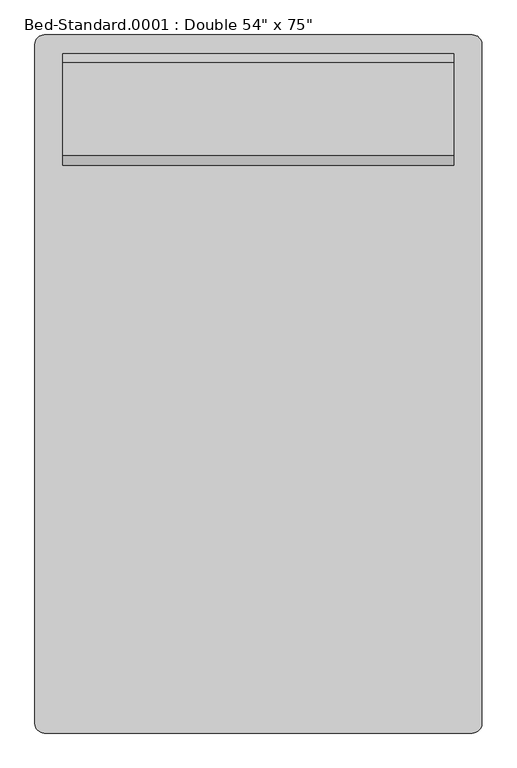
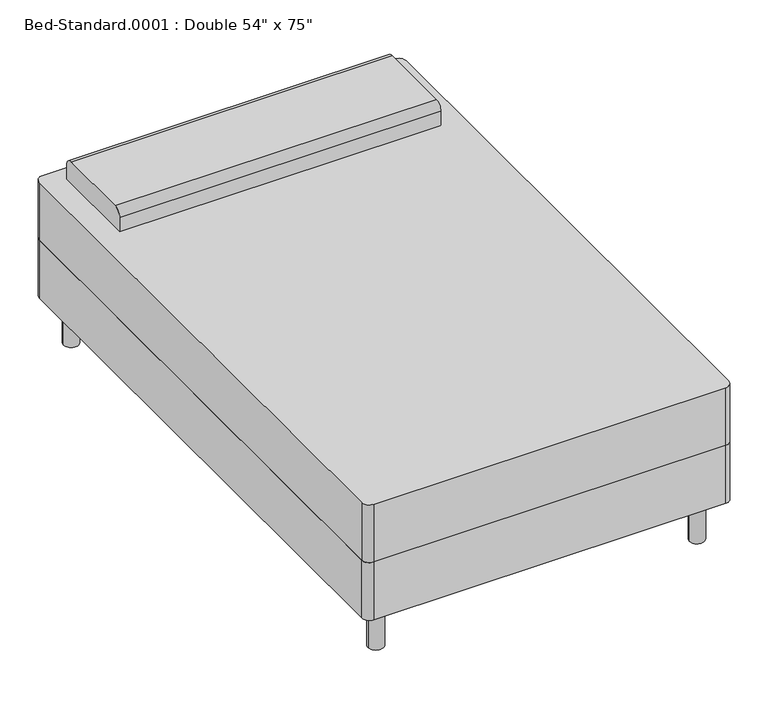
"""IFC4 building model written with IfcOpenShell, lengths in millimetres: furniture geometry."""

from ifc_helpers import new_model, si_unit, point, frame, frame_2d, origin, origin_with_axes, place, context, project, spatial, polyline, circle_curve, trimmed, segment, composite_curve, outline, extrude, source, transform, mapped, element, save


def furniture_4e05012c(model_context):
    return source(origin(), model_context, "Body", "SweptSolid", [
        extrude(outline(composite_curve([segment(polyline([(-338.1114754, -972.695082), (-338.1114754, 881.504918)]), True, "CONTINUOUS"), segment(trimmed(circle_curve(frame_2d((-312.7114754, 881.504918)), 25.4), [point((-338.1114754, 881.504918))], [point((-312.7114754, 906.904918))], False, "CARTESIAN"), True, "CONTINUOUS"), segment(polyline([(-312.7114754, 906.904918), (855.6885246, 906.904918)]), True, "CONTINUOUS"), segment(trimmed(circle_curve(frame_2d((855.6885246, 881.504918)), 25.4), [point((855.6885246, 906.904918))], [point((881.0885246, 881.504918))], False, "CARTESIAN"), True, "CONTINUOUS"), segment(polyline([(881.0885246, 881.504918), (881.0885246, -972.695082)]), True, "CONTINUOUS"), segment(trimmed(circle_curve(frame_2d((855.6885246, -972.695082)), 25.4), [point((881.0885246, -972.695082))], [point((855.6885246, -998.095082))], False, "CARTESIAN"), True, "CONTINUOUS"), segment(polyline([(855.6885246, -998.095082), (-312.7114754, -998.095082)]), True, "CONTINUOUS"), segment(trimmed(circle_curve(frame_2d((-312.7114754, -972.695082)), 25.4), [point((-312.7114754, -998.095082))], [point((-338.1114754, -972.695082))], False, "CARTESIAN"), True, "CONTINUOUS")], self_intersect=False)), frame((0.0, 0.0, 152.4), z_axis=(0.0, 0.0, 1.0), x_axis=(1.0, 0.0, 0.0)), (0.0, 0.0, 1.0), 203.2),
        extrude(outline(composite_curve([segment(polyline([(551.304918, 558.8), (551.304918, 609.6)]), True, "CONTINUOUS"), segment(trimmed(circle_curve(frame_2d((576.704918, 609.6)), 25.4), [point((551.304918, 609.6))], [point((576.704918, 635.0))], False, "CARTESIAN"), True, "CONTINUOUS"), segment(polyline([(576.704918, 635.0), (830.704918, 635.0)]), True, "CONTINUOUS"), segment(trimmed(circle_curve(frame_2d((830.704918, 609.6)), 25.4), [point((830.704918, 635.0))], [point((856.104918, 609.6))], False, "CARTESIAN"), True, "CONTINUOUS"), segment(polyline([(856.104918, 609.6), (856.104918, 558.8), (551.304918, 558.8)]), True, "CONTINUOUS")], self_intersect=False)), frame((-261.9114754, 0.0, 0.0), z_axis=(1.0, 0.0, 0.0), x_axis=(0.0, 1.0, 0.0)), (0.0, 0.0, 1.0), 1066.8),
        extrude(outline(composite_curve([segment(trimmed(circle_curve(frame_2d((-261.9114754, 830.704918)), 25.4), [point((-287.3114754, 830.704918))], [point((-236.5114754, 830.704918))], False, "CARTESIAN"), True, "CONTINUOUS"), segment(trimmed(circle_curve(frame_2d((-261.9114754, 830.704918)), 25.4), [point((-236.5114754, 830.704918))], [point((-287.3114754, 830.704918))], False, "CARTESIAN"), True, "CONTINUOUS")], self_intersect=False)), origin_with_axes(), (0.0, 0.0, 1.0), 152.4),
        extrude(outline(composite_curve([segment(trimmed(circle_curve(frame_2d((804.8885246, 830.704918)), 25.4), [point((779.4885246, 830.704918))], [point((830.2885246, 830.704918))], False, "CARTESIAN"), True, "CONTINUOUS"), segment(trimmed(circle_curve(frame_2d((804.8885246, 830.704918)), 25.4), [point((830.2885246, 830.704918))], [point((779.4885246, 830.704918))], False, "CARTESIAN"), True, "CONTINUOUS")], self_intersect=False)), origin_with_axes(), (0.0, 0.0, 1.0), 152.4),
        extrude(outline(composite_curve([segment(trimmed(circle_curve(frame_2d((804.8885246, -921.895082)), 25.4), [point((779.4885246, -921.895082))], [point((830.2885246, -921.895082))], False, "CARTESIAN"), True, "CONTINUOUS"), segment(trimmed(circle_curve(frame_2d((804.8885246, -921.895082)), 25.4), [point((830.2885246, -921.895082))], [point((779.4885246, -921.895082))], False, "CARTESIAN"), True, "CONTINUOUS")], self_intersect=False)), origin_with_axes(), (0.0, 0.0, 1.0), 152.4),
        extrude(outline(composite_curve([segment(trimmed(circle_curve(frame_2d((-261.9114754, -921.895082)), 25.4), [point((-287.3114754, -921.895082))], [point((-236.5114754, -921.895082))], False, "CARTESIAN"), True, "CONTINUOUS"), segment(trimmed(circle_curve(frame_2d((-261.9114754, -921.895082)), 25.4), [point((-236.5114754, -921.895082))], [point((-287.3114754, -921.895082))], False, "CARTESIAN"), True, "CONTINUOUS")], self_intersect=False)), origin_with_axes(), (0.0, 0.0, 1.0), 152.4),
        extrude(outline(composite_curve([segment(polyline([(-312.7114754, 906.904918), (855.6885246, 906.904918)]), True, "CONTINUOUS"), segment(trimmed(circle_curve(frame_2d((855.6885246, 881.504918)), 25.4), [point((855.6885246, 906.904918))], [point((881.0885246, 881.504918))], False, "CARTESIAN"), True, "CONTINUOUS"), segment(polyline([(881.0885246, 881.504918), (881.0885246, -972.695082)]), True, "CONTINUOUS"), segment(trimmed(circle_curve(frame_2d((855.6885246, -972.695082)), 25.4), [point((881.0885246, -972.695082))], [point((855.6885246, -998.095082))], False, "CARTESIAN"), True, "CONTINUOUS"), segment(polyline([(855.6885246, -998.095082), (-312.7114754, -998.095082)]), True, "CONTINUOUS"), segment(trimmed(circle_curve(frame_2d((-312.7114754, -972.695082)), 25.4), [point((-312.7114754, -998.095082))], [point((-338.1114754, -972.695082))], False, "CARTESIAN"), True, "CONTINUOUS"), segment(polyline([(-338.1114754, -972.695082), (-338.1114754, 881.504918)]), True, "CONTINUOUS"), segment(trimmed(circle_curve(frame_2d((-312.7114754, 881.504918)), 25.4), [point((-338.1114754, 881.504918))], [point((-312.7114754, 906.904918))], False, "CARTESIAN"), True, "CONTINUOUS")], self_intersect=False)), frame((0.0, 0.0, 355.6), z_axis=(0.0, 0.0, 1.0), x_axis=(1.0, 0.0, 0.0)), (0.0, 0.0, 1.0), 203.2),
    ])


if __name__ == "__main__":
    model = new_model("IFC4")
    model_context = context("Model", 3, world=origin())
    ifc_project = project(units=[si_unit("LENGTHUNIT", "METRE", prefix="MILLI")], contexts=[model_context])
    site = spatial("IfcSite", under=ifc_project)
    building = spatial("IfcBuilding", under=site)
    placement = place(None, origin())
    furniture_shape = furniture_4e05012c(model_context)
    element("IfcFurniture", 1, ObjectType="Bed-Standard.0001 : Double 54\" x 75\"", at=placement, inside=building, context=model_context, shape_type="MappedRepresentation", body=[
        mapped(furniture_shape, transform((0.0, 0.0, 0.0), x_axis=(1.0, 0.0, 0.0), y_axis=(0.0, 1.0, 0.0), z_axis=(0.0, 0.0, 1.0))),
    ])
    save(model, "model.ifc")

# Revit data of these elements
# Type "Bed-Standard.0001 : Double 54\" x 75\""
#   Assembly Code = "E2020200"
#   Length = 6' - 3"
#   Width = 4' - 0"
#   Leg Material = Steel, Chrome Plated
#   Mattress Material = Linen, White
#   Default Elevation = 0
# Element 1 (IfcFurniture, "Bed-Standard.0001 : Double 54\" x 75\"")
#   Materials on its faces: "Linen, White", "Steel, Chrome Plated"
# Materials
#   "Steel, Chrome Plated": class "Metal", colour RGB 17 17 17, transparency 0, Description = "Chromiuim plated steel", Cost = 0
#   "Linen, White": class "Textile", colour RGB 247 247 239, transparency 0, Description = "Linen, white", Cost = 0
